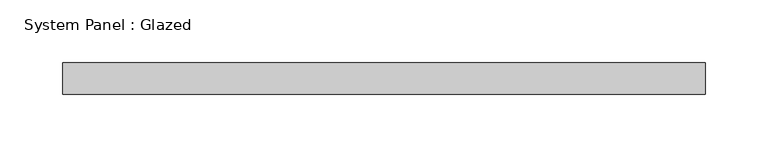
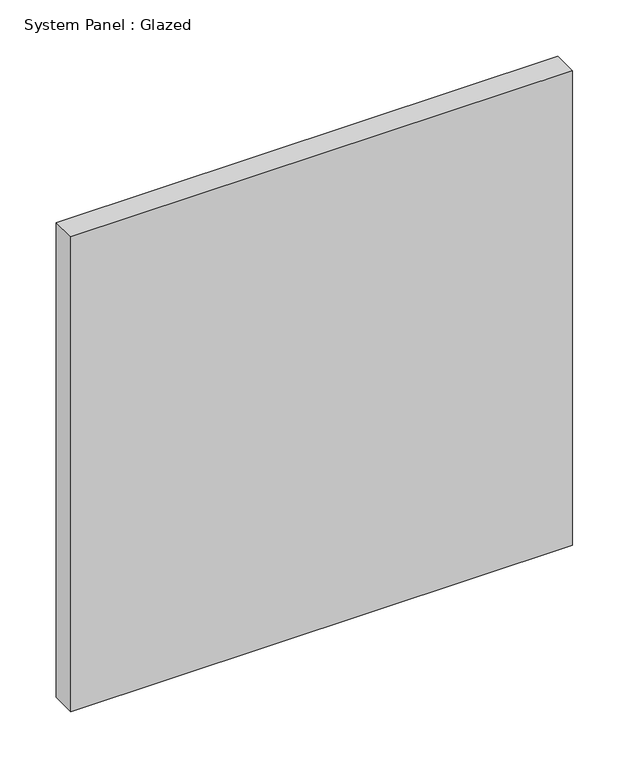
"""IFC4 building model written with IfcOpenShell, lengths in millimetres: plate geometry, System Panel : Glazed."""

from ifc_helpers import new_model, si_unit, origin, origin_with_axes, place, context, project, spatial, polyline, outline, extrude, source, transform, mapped, element, save


def system_panel_glazed_c086748d(model_context):
    return source(origin(), model_context, "Body", "SweptSolid", [
        extrude(outline(polyline([(257.175, 19.05), (-257.175, 19.05), (-257.175, 44.45), (257.175, 44.45), (257.175, 19.05)])), origin_with_axes(), (0.0, 0.0, 1.0), 514.35),
    ])


if __name__ == "__main__":
    model = new_model("IFC4")
    model_context = context("Model", 3, world=origin())
    ifc_project = project(units=[si_unit("LENGTHUNIT", "METRE", prefix="MILLI")], contexts=[model_context])
    site = spatial("IfcSite", under=ifc_project)
    building = spatial("IfcBuilding", under=site)
    placement = place(None, origin())
    system_panel_glazed_shape = system_panel_glazed_c086748d(model_context)
    element("IfcPlate", 1, ObjectType="System Panel : Glazed", at=placement, inside=building, context=model_context, shape_type="MappedRepresentation", body=[
        mapped(system_panel_glazed_shape, transform((0.0, 0.0, 0.0), x_axis=(1.0, 0.0, 0.0), y_axis=(0.0, 1.0, 0.0), z_axis=(0.0, 0.0, 1.0))),
    ])
    save(model, "model.ifc")

# Revit data of these elements
# Type "System Panel : Glazed"
#   Construction Type Id = "GSP4R"
#   Analytic Construction = "1/8 in Pilkington single glazing"
#   Visual Light Transmittance = 0.9
#   Solar Heat Gain Coefficient = 0.86
#   Heat Transfer Coefficient (U) = 1.18115 BTU/(h·ft²·°F)
#   Define Thermal Properties by = 1
# Element 1 (IfcPlate, "System Panel : Glazed")
#   Materials on its faces: "Glass"
# Materials
#   "Glass": class "Glass", colour RGB 0 128 192, transparency 0.75, Description = "Soda Lime Glass", Cost = 0
